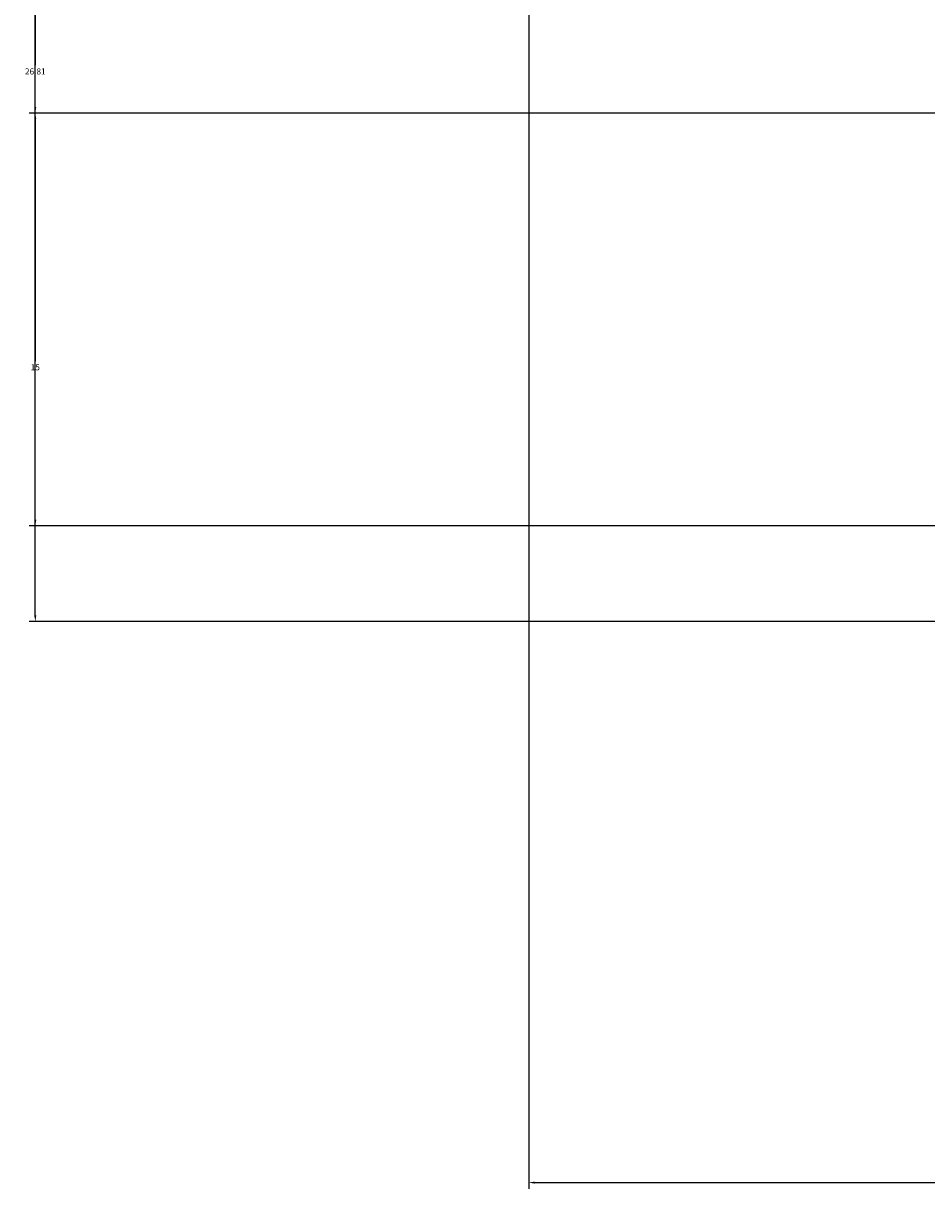
# Model space of a CAD drawing. Units: inches. Extents: x -12 to 334, y -10 to 186.
# Tile 1 of 77: x -12 to 15, y 14 to 49. Entities that reach past the tile are written whole.
import ezdxf

# ---------------------------------------------------------------- set-up
doc = ezdxf.new("R2010")
doc.units = ezdxf.units.IN
doc.header["$MEASUREMENT"] = 0
doc.layers.add('M-DIMS', color=2, linetype='Continuous', lineweight=18)
doc.styles.get("Standard").update_dxf_attribs({"font": 'arial.ttf'})
doc.dimstyles.get("Standard").update_dxf_attribs({"dimtxt": 0.18, "dimasz": 0.18, "dimexe": 0.18, "dimexo": 0.0625, "dimgap": 0.09, "dimtad": 0, "dimtih": 1, "dimtoh": 1, "dimdec": 4, "dimzin": 0, "dimdsep": 46, "dimtxsty": 'Standard', "dimcen": 0.09, "dimadec": 0, "dimazin": 0, "dimtfac": 1, "dimtdec": 4, "dimtofl": 0, "dimtmove": 0, "dimatfit": 3, "dimfxl": 1, "dimtolj": 1, "dimtzin": 0, "dimarcsym": 0})

# ---------------------------------------------------------------- blocks, each defined once
blk = doc.blocks.new('*D1')
at = {"layer": 'Defpoints', "color": 0, "transparency": 16777216}
for p in [(281.426, 91.899), (3.376, 80.692), (281.426, 14.304)]:
    blk.add_point(p, dxfattribs=at)
at = {"layer": 'M-DIMS', "color": 0, "lineweight": -2, "transparency": 16777216}
for p, q in [((281.426, 91.836), (281.426, 14.124)), ((3.376, 80.629), (3.376, 14.124)), ((3.556, 14.304), (141.935, 14.304)), ((281.246, 14.304), (142.867, 14.304))]:
    blk.add_line(p, q, dxfattribs=at)
at = {"layer": 'M-DIMS', "color": 0, "transparency": 16777216}
for points in [[(3.556, 14.334), (3.556, 14.274), (3.376, 14.304)], [(281.246, 14.334), (281.246, 14.274), (281.426, 14.304)]]:
    blk.add_solid(points, dxfattribs=at)
at = {"layer": 'M-DIMS', "color": 0, "transparency": 16777216, "insert": (142.401, 14.304), "char_height": 0.18, "attachment_point": 5}
blk.add_mtext('\\A1;278.05', dxfattribs=at)
blk = doc.blocks.new('*D6')
at = {"layer": 'Defpoints', "color": 0, "transparency": 16777216}
for p in [(-11.174, 60.487), (23.581, 60.487), (32.1, 33.675)]:
    blk.add_point(p, dxfattribs=at)
at = {"layer": 'M-DIMS', "color": 0, "lineweight": -2, "transparency": 16777216}
for p, q in [((23.518, 60.487), (-11.354, 60.487)), ((-11.174, 60.307), (-11.174, 47.263)), ((-11.174, 33.855), (-11.174, 46.899)), ((32.038, 33.675), (-11.354, 33.675))]:
    blk.add_line(p, q, dxfattribs=at)
at = {"layer": 'M-DIMS', "color": 0, "transparency": 16777216}
for points in [[(-11.204, 60.307), (-11.144, 60.307), (-11.174, 60.487)], [(-11.204, 33.855), (-11.144, 33.855), (-11.174, 33.675)]]:
    blk.add_solid(points, dxfattribs=at)
at = {"layer": 'M-DIMS', "color": 0, "transparency": 16777216, "insert": (-11.174, 47.081), "char_height": 0.18, "attachment_point": 5}
blk.add_mtext('\\A1;26.81', dxfattribs=at)
blk = doc.blocks.new('*D29')
at = {"layer": 'Defpoints', "color": 0, "transparency": 16777216}
for p in [(-11.174, 45.854), (221.576, 45.854), (216.576, 30.854)]:
    blk.add_point(p, dxfattribs=at)
at = {"layer": 'M-DIMS', "color": 0, "lineweight": -2, "transparency": 16777216}
for p, q in [((221.514, 45.854), (-11.354, 45.854)), ((-11.174, 45.674), (-11.174, 38.536)), ((-11.174, 31.034), (-11.174, 38.172)), ((216.514, 30.854), (-11.354, 30.854))]:
    blk.add_line(p, q, dxfattribs=at)
at = {"layer": 'M-DIMS', "color": 0, "transparency": 16777216}
for points in [[(-11.204, 45.674), (-11.144, 45.674), (-11.174, 45.854)], [(-11.204, 31.034), (-11.144, 31.034), (-11.174, 30.854)]]:
    blk.add_solid(points, dxfattribs=at)
at = {"layer": 'M-DIMS', "color": 0, "transparency": 16777216, "insert": (-11.174, 38.354), "char_height": 0.18, "attachment_point": 5}
blk.add_mtext('\\A1;15', dxfattribs=at)
blk = doc.blocks.new('*D39')
at = {"layer": 'Defpoints', "color": 0, "transparency": 16777216}
for p in [(279.726, 80.692), (-11.174, 45.854), (269.381, 45.854)]:
    blk.add_point(p, dxfattribs=at)
at = {"layer": 'M-DIMS', "color": 0, "lineweight": -2, "transparency": 16777216}
for p, q in [((279.664, 80.692), (-11.354, 80.692)), ((-11.174, 80.512), (-11.174, 63.455)), ((-11.174, 46.034), (-11.174, 63.091)), ((269.318, 45.854), (-11.354, 45.854))]:
    blk.add_line(p, q, dxfattribs=at)
at = {"layer": 'M-DIMS', "color": 0, "transparency": 16777216}
for points in [[(-11.204, 80.512), (-11.144, 80.512), (-11.174, 80.692)], [(-11.204, 46.034), (-11.144, 46.034), (-11.174, 45.854)]]:
    blk.add_solid(points, dxfattribs=at)
at = {"layer": 'M-DIMS', "color": 0, "transparency": 16777216, "insert": (-11.174, 63.273), "char_height": 0.18, "attachment_point": 5}
blk.add_mtext('\\A1;34.84', dxfattribs=at)

msp = doc.modelspace()

# ---------------------------------------------------------------- dimensions: what is measured, and where the dimension line sits
at = {"layer": 'M-DIMS'}
dim = msp.add_linear_dim(base=(281.4256, 14.3041), p1=(3.3765, 80.6915), p2=(281.4256, 91.8988), dimstyle='Standard', override={"dimdec": 2, "dimlfac": 1, "dimrnd": 0, "dimzin": 0, "dimdsep": 46, "dimlunit": 2}, dxfattribs=at)
dim.commit()
dim.dimension.update_dxf_attribs({"geometry": '*D1', "text_midpoint": (142.401, 14.3041)})
for base, p1, p2, override, picture, middle in [((-11.1736, 45.8541), (279.7263, 80.6915), (269.3808, 45.8541), {"dimdec": 2, "dimlfac": 1, "dimrnd": 0, "dimzin": 0, "dimdsep": 46, "dimlunit": 2}, '*D39', (-11.1735, 63.2728)), ((-11.1736, 60.4872), (32.1002, 33.6752), (23.5807, 60.4872), {"dimdec": 2, "dimlfac": 1, "dimrnd": 0, "dimzin": 0, "dimdsep": 46, "dimlunit": 2}, '*D6', (-11.1735, 47.0812)), ((-11.1736, 45.8541), (216.5761, 30.8541), (221.5761, 45.8541), {"dimdec": 0, "dimlfac": 1, "dimrnd": 0, "dimzin": 0, "dimdsep": 46, "dimlunit": 2}, '*D29', (-11.1735, 38.3541))]:
    dim = msp.add_linear_dim(base=base, p1=p1, p2=p2, angle=90, dimstyle='Standard', override=override, dxfattribs=at)
    dim.commit()
    dim.dimension.update_dxf_attribs({"geometry": picture, "text_midpoint": middle})

doc.saveas('drawing.dxf')
